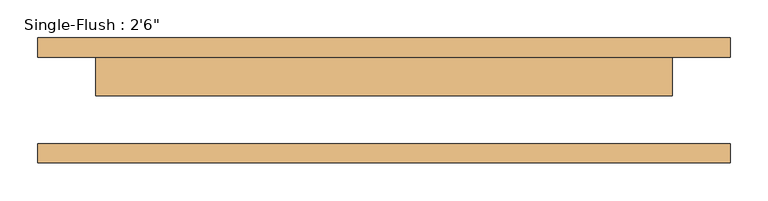
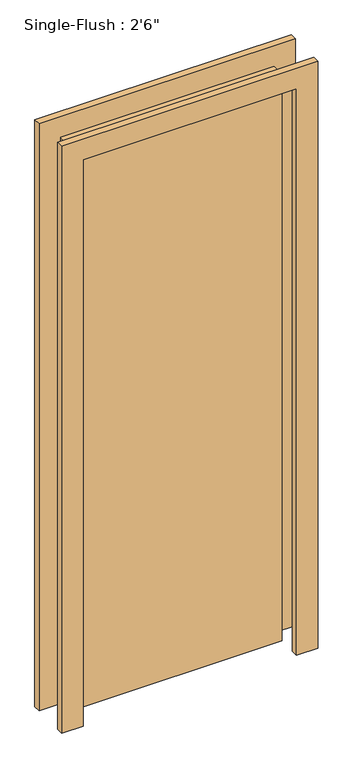
"""IFC4 building model written with IfcOpenShell, lengths in millimetres: door geometry."""

from ifc_helpers import new_model, si_unit, frame, origin, origin_with_axes, place, context, project, spatial, polyline, outline, extrude, source, transform, mapped, element, save


def door_214872d5(model_context):
    return source(origin(), model_context, "Body", "SweptSolid", [
        extrude(outline(polyline([(2209.8, -457.2), (0.0, -457.2), (0.0, -381.0), (2133.6, -381.0), (2133.6, 381.0), (0.0, 381.0), (0.0, 457.2), (2209.8, 457.2), (2209.8, -457.2)])), frame((0.0, 57.15, 0.0), z_axis=(0.0, 1.0, 0.0), x_axis=(0.0, 0.0, 1.0)), (0.0, 0.0, 1.0), 25.4),
        extrude(outline(polyline([(2209.8, 457.2), (2209.8, -457.2), (0.0, -457.2), (0.0, -381.0), (2133.6, -381.0), (2133.6, 381.0), (0.0, 381.0), (0.0, 457.2), (2209.8, 457.2)])), frame((0.0, -82.55, 0.0), z_axis=(0.0, 1.0, 0.0), x_axis=(0.0, 0.0, 1.0)), (0.0, 0.0, 1.0), 25.4),
        extrude(outline(polyline([(381.0, 6.35), (-381.0, 6.35), (-381.0, 57.15), (381.0, 57.15), (381.0, 6.35)])), origin_with_axes(), (0.0, 0.0, 1.0), 2133.6),
    ])


if __name__ == "__main__":
    model = new_model("IFC4")
    model_context = context("Model", 3, world=origin())
    ifc_project = project(units=[si_unit("LENGTHUNIT", "METRE", prefix="MILLI")], contexts=[model_context])
    site = spatial("IfcSite", under=ifc_project)
    building = spatial("IfcBuilding", under=site)
    placement = place(None, origin())
    door_shape = door_214872d5(model_context)
    element("IfcDoor", 1, ObjectType="Single-Flush : 2'6\"", at=placement, inside=building, context=model_context, shape_type="MappedRepresentation", body=[
        mapped(door_shape, transform((0.0, 0.0, 0.0), x_axis=(1.0, 0.0, 0.0), y_axis=(0.0, 1.0, 0.0), z_axis=(0.0, 0.0, 1.0))),
    ])
    save(model, "model.ifc")

# Revit data of these elements
# Type "Single-Flush : 2'6\""
#   Type Mark = "9"
#   Construction Type Id = "MDOOR"
#   Assembly Code = "C1020"
#   Analytic Construction = "Metal"
#   Thickness = 0' - 2"
#   Heat Transfer Coefficient (U) = 0.651978 BTU/(h·ft²·°F)
#   Height = 7' - 0"
#   Trim Projection Ext = 0' - 1"
#   Trim Projection Int = 0' - 1"
#   Trim Width = 0' - 3"
#   Width = 2' - 6"
#   Define Thermal Properties by = 1
#   Door Material = Door - Panel
#   Frame Material = Door - Frame
#   Visual Light Transmittance = 0
#   Solar Heat Gain Coefficient = 0
#   Function = (empty or 0)
#   Wall Closure = (empty or 0)
# Element 1 (IfcDoor, "Single-Flush : 2'6\"")
#   Materials on its faces: "Door - Frame", "Door - Panel"
# Materials
#   "Door - Panel": class "Wood", colour RGB 210 159 95, transparency 0, Cost = 0
#   "Door - Frame": colour RGB 118 70 51, transparency 0, Cost = 0
